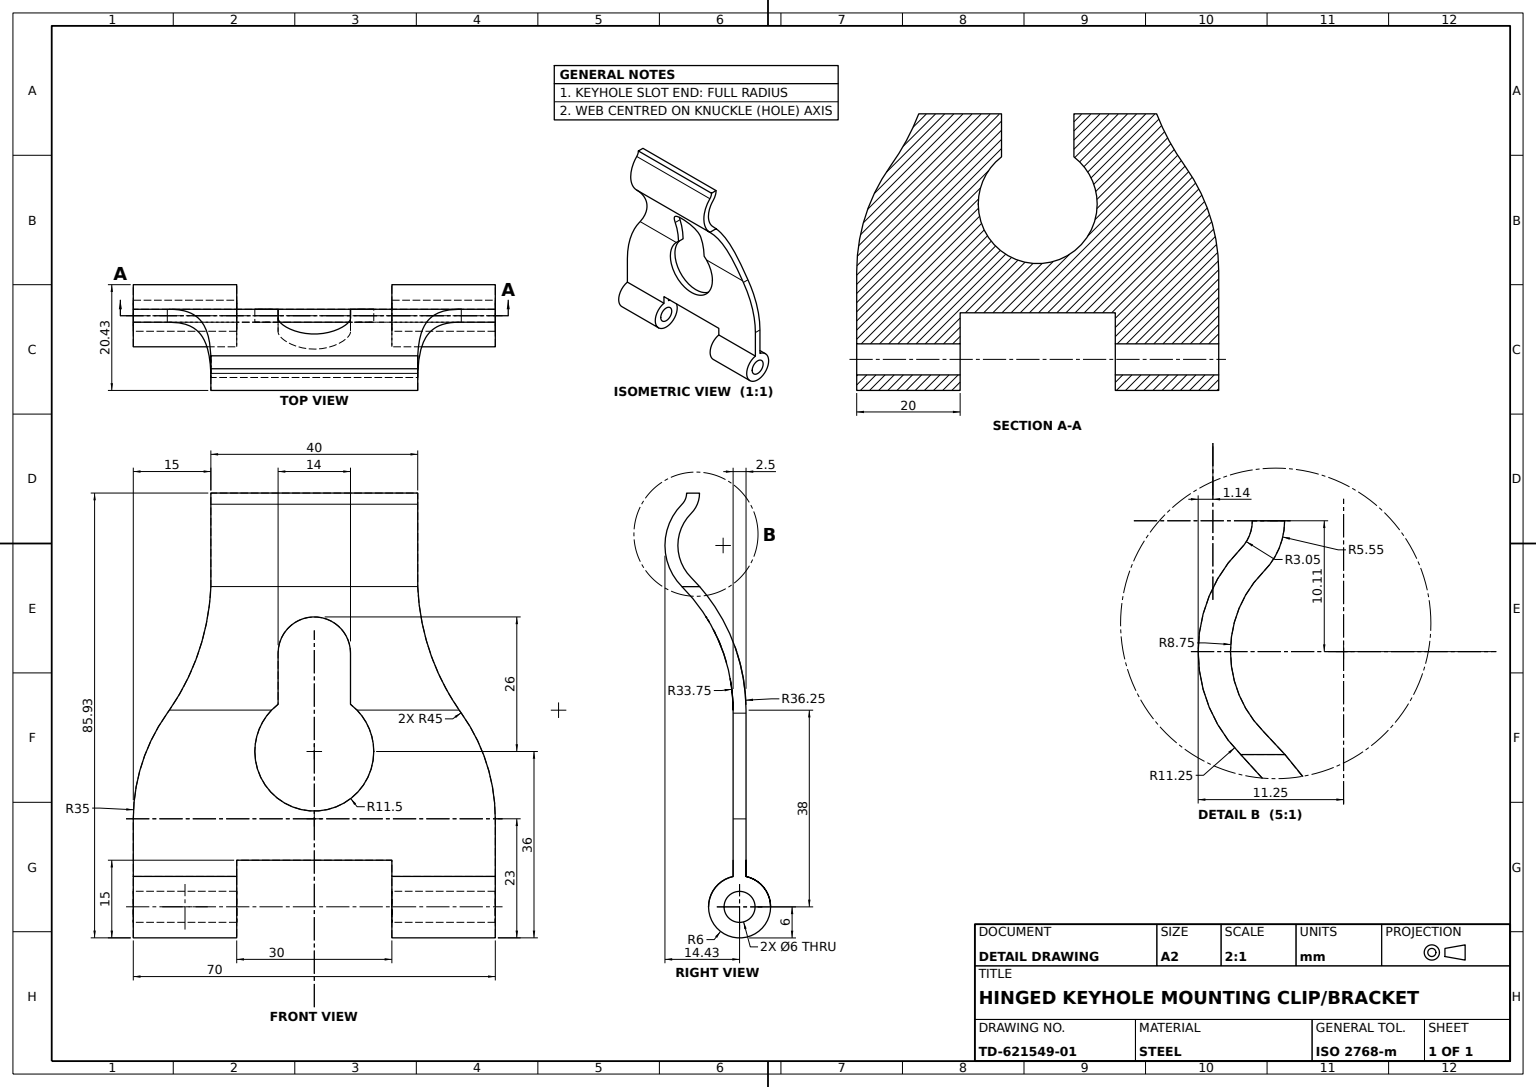
from build123d import *

# Parameters (mm, degrees)
BRACKET_SIDE_PROFILE_SKETCH_R        = 3
BRACKET_BODY_EXTRUDE_70MM_DEPTH      = 35
OUTLINE_AND_KEYHOLE_CUT_DEPTH        = 89.24823725
OUTLINE_AND_KEYHOLE_CUT_DEPTH_BACK   = 89.24823725
OUTLINE_AND_KEYHOLE_SKETCH_OUTSIDE_W = 94.54
OUTLINE_AND_KEYHOLE_SKETCH_OUTSIDE_H = 110.471


with BuildPart() as part:
    # Bracket Side Profile Sketch → Bracket Body Extrude 70mm (new, symmetric)
    with BuildSketch(Plane(origin=(0, 0, 0), x_dir=(0, 0, -1), z_dir=(1, 0, 0))):
        with BuildLine():
            Line((1.25, 5.868347297), (1.25, 38))
            ThreePointArc((1.25, 38), (-1.509366946, 51.872274423), (-9.367379182, 63.632620818))
            ThreePointArc((-9.367379182, 63.632620818), (-11.930194847, 69.819805153), (-9.367379182, 76.006989489))
            ThreePointArc((-9.367379182, 76.006989489), (-8.164290412, 77.807539075), (-7.741821818, 79.931432124))
            Line((-7.741821818, 79.931432124), (-10.241821818, 79.931432124))
            ThreePointArc((-10.241821818, 79.931432124), (-10.473989243, 78.764247656), (-11.135146135, 77.774756442))
            ThreePointArc((-11.135146135, 77.774756442), (-14.430194847, 69.819805153), (-11.135146135, 61.864853865))
            ThreePointArc((-11.135146135, 61.864853865), (-3.819065778, 50.915565842), (-1.25, 38))
            Line((-1.25, 38), (-1.25, 5.868347297))
            ThreePointArc((-1.25, 5.868347297), (0, -6), (1.25, 5.868347297))
        make_face()
        Circle(BRACKET_SIDE_PROFILE_SKETCH_R, mode=Mode.SUBTRACT)
    extrude(amount=BRACKET_BODY_EXTRUDE_70MM_DEPTH, both=True)

    # Outline and Keyhole Sketch outside → Outline and Keyhole Cut (cut, two sides: drawn at the far end of the back side and taken through both)
    # profile 1 of 2: a face of its own
    with BuildSketch(Plane.XY.offset(1.25).offset(-OUTLINE_AND_KEYHOLE_CUT_DEPTH_BACK)):
        with Locations((0, 36.9655)):
            Rectangle(OUTLINE_AND_KEYHOLE_SKETCH_OUTSIDE_W, OUTLINE_AND_KEYHOLE_SKETCH_OUTSIDE_H)
        with BuildLine():
            Line((35, -6), (35, 17))
            ThreePointArc((35, 17), (33.314760402, 27.729712921), (28.421329179, 37.426160865))
            ThreePointArc((28.421329179, 37.426160865), (22.418139751, 49.027821234), (20, 61.864853865))
            Line((20, 61.864853865), (20, 79.931432124))
            Line((20, 79.931432124), (-20, 79.931432124))
            Line((-20, 79.931432124), (-20, 61.864853865))
            ThreePointArc((-20, 61.864853865), (-22.418139751, 49.027821234), (-28.421329179, 37.426160865))
            ThreePointArc((-28.421329179, 37.426160865), (-33.314760402, 27.729712921), (-35, 17))
            Line((-35, 17), (-35, -6))
            Line((-35, -6), (-15, -6))
            Line((-15, -6), (-15, 9))
            Line((-15, 9), (15, 9))
            Line((15, 9), (15, -6))
            Line((15, -6), (35, -6))
        make_face(mode=Mode.SUBTRACT)
    # profile 2 of 2: a face of its own
    with BuildSketch(Plane.XY.offset(1.25).offset(-OUTLINE_AND_KEYHOLE_CUT_DEPTH_BACK)):
        with BuildLine():
            Line((7, 49), (7, 39.124143795))
            ThreePointArc((7, 39.124143795), (0, 18.5), (-7, 39.124143795))
            Line((-7, 39.124143795), (-7, 49))
            ThreePointArc((-7, 49), (0, 56), (7, 49))
        make_face()
    extrude(amount=OUTLINE_AND_KEYHOLE_CUT_DEPTH + OUTLINE_AND_KEYHOLE_CUT_DEPTH_BACK, mode=Mode.SUBTRACT)


solid = part.part
